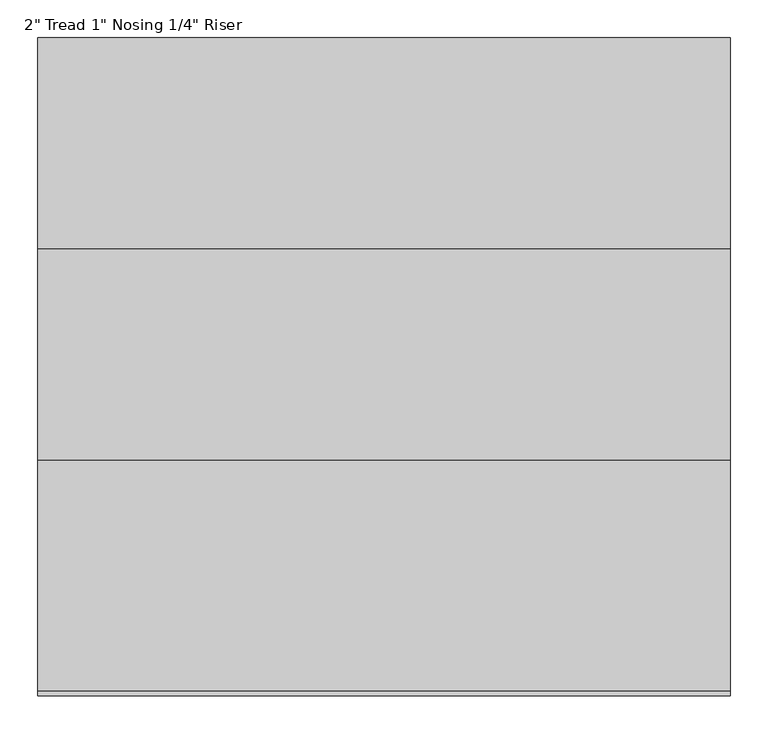
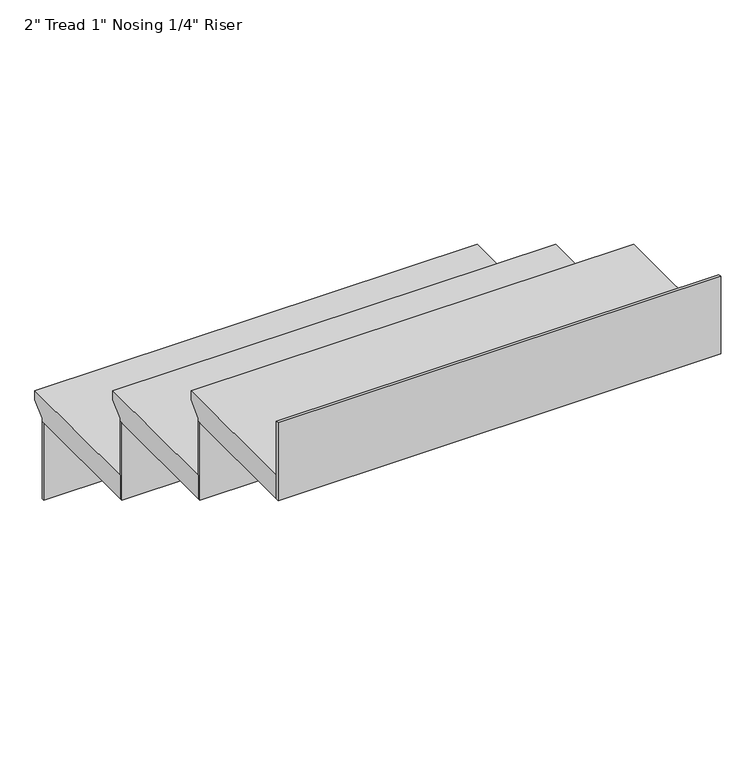
"""IFC4 building model written with IfcOpenShell, lengths in millimetres: stair flight geometry."""

from ifc_helpers import new_model, si_unit, frame, origin, place, context, project, spatial, polyline, outline, extrude, source, transform, mapped, element, save


def stair_flight_7c360194(model_context):
    return source(origin(), model_context, "Body", "SweptSolid", [
        extrude(outline(polyline([(-19826.9851539, 27774.6172466), (-19522.1851539, 27774.6172466), (-19522.1851539, 27755.5672466), (-19547.5851539, 27730.1672466), (-19547.5851539, 27723.8172466), (-19826.9851539, 27723.8172466), (-19826.9851539, 27774.6172466)])), frame((-2296.6415084, 0.0, 0.0), z_axis=(1.0, 0.0, 0.0), x_axis=(0.0, 1.0, 0.0)), (0.0, 0.0, 1.0), 914.4),
        extrude(outline(polyline([(-2296.6415084, -19553.9351539), (-2296.6415084, -19547.5851539), (-1382.2415084, -19547.5851539), (-1382.2415084, -19553.9351539), (-2296.6415084, -19553.9351539)])), frame((0.0, 0.0, 27554.4839133), z_axis=(0.0, 0.0, 1.0), x_axis=(1.0, 0.0, 0.0)), (0.0, 0.0, 1.0), 169.3333333),
        extrude(outline(polyline([(-2296.6415084, -19833.3351539), (-2296.6415084, -19826.9851539), (-1382.2415084, -19826.9851539), (-1382.2415084, -19833.3351539), (-2296.6415084, -19833.3351539)])), frame((0.0, 0.0, 27723.8172466), z_axis=(0.0, 0.0, 1.0), x_axis=(1.0, 0.0, 0.0)), (0.0, 0.0, 1.0), 169.3333333),
        extrude(outline(polyline([(-20106.3851539, 27943.9505799), (-19801.5851539, 27943.9505799), (-19801.5851539, 27924.9005799), (-19826.9851539, 27899.5005799), (-19826.9851539, 27893.1505799), (-20106.3851539, 27893.1505799), (-20106.3851539, 27943.9505799)])), frame((-2296.6415084, 0.0, 0.0), z_axis=(1.0, 0.0, 0.0), x_axis=(0.0, 1.0, 0.0)), (0.0, 0.0, 1.0), 914.4),
        extrude(outline(polyline([(-2296.6415084, -20112.7351539), (-2296.6415084, -20106.3851539), (-1382.2415084, -20106.3851539), (-1382.2415084, -20112.7351539), (-2296.6415084, -20112.7351539)])), frame((0.0, 0.0, 27893.1505799), z_axis=(0.0, 0.0, 1.0), x_axis=(1.0, 0.0, 0.0)), (0.0, 0.0, 1.0), 169.3333333),
        extrude(outline(polyline([(-2296.6415084, -20392.1351539), (-2296.6415084, -20385.7851539), (-1382.2415084, -20385.7851539), (-1382.2415084, -20392.1351539), (-2296.6415084, -20392.1351539)])), frame((0.0, 0.0, 28062.4839133), z_axis=(0.0, 0.0, 1.0), x_axis=(1.0, 0.0, 0.0)), (0.0, 0.0, 1.0), 169.3333333),
        extrude(outline(polyline([(-20385.7851539, 28113.2839133), (-20080.9851539, 28113.2839133), (-20080.9851539, 28094.2339133), (-20106.3851539, 28068.8339133), (-20106.3851539, 28062.4839133), (-20385.7851539, 28062.4839133), (-20385.7851539, 28113.2839133)])), frame((-2296.6415084, 0.0, 0.0), z_axis=(1.0, 0.0, 0.0), x_axis=(0.0, 1.0, 0.0)), (0.0, 0.0, 1.0), 914.4),
    ])


if __name__ == "__main__":
    model = new_model("IFC4")
    model_context = context("Model", 3, world=origin())
    ifc_project = project(units=[si_unit("LENGTHUNIT", "METRE", prefix="MILLI")], contexts=[model_context])
    site = spatial("IfcSite", under=ifc_project)
    building = spatial("IfcBuilding", under=site)
    placement = place(None, origin())
    stair_flight_shape = stair_flight_7c360194(model_context)
    element("IfcStairFlight", 1, ObjectType="2\" Tread 1\" Nosing 1/4\" Riser", at=placement, inside=building, context=model_context, shape_type="MappedRepresentation", body=[
        mapped(stair_flight_shape, transform((0.0, 0.0, 0.0), x_axis=(1.0, 0.0, 0.0), y_axis=(0.0, 1.0, 0.0), z_axis=(0.0, 0.0, 1.0))),
    ])
    save(model, "model.ifc")
